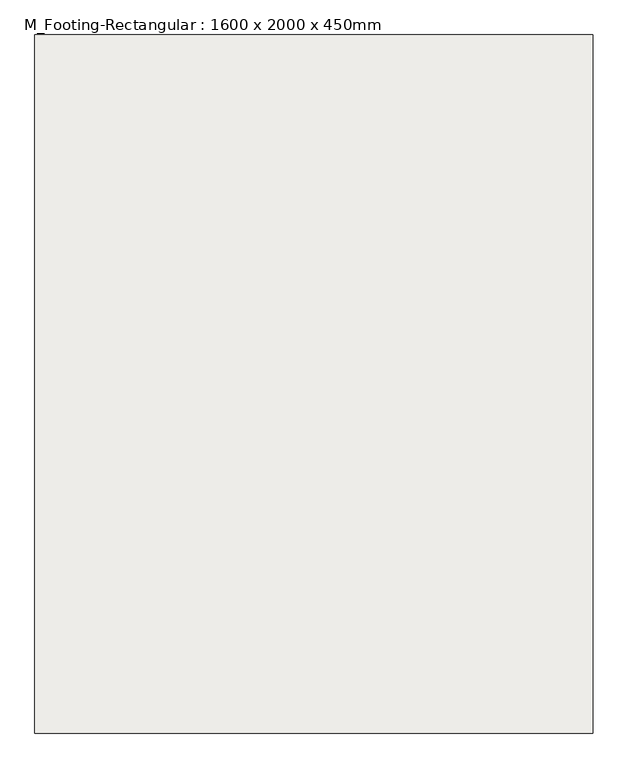
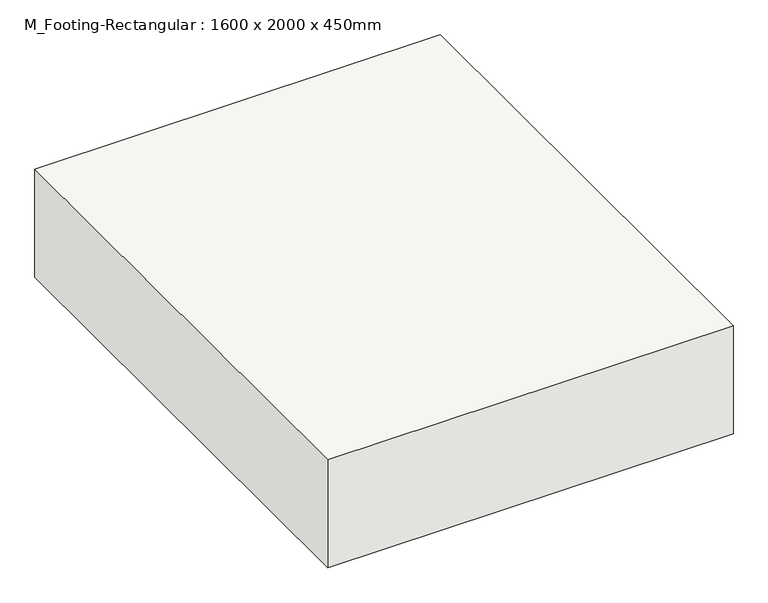
"""IFC4 building model written with IfcOpenShell, lengths in millimetres: slab geometry, M_Footing-Rectangular : 1600 x 2000 x 450mm."""

from ifc_helpers import new_model, si_unit, frame, origin, place, context, project, spatial, polyline, outline, extrude, source, transform, mapped, element, save


def m_footing_rectangular_1600_x_2000_x_450mm_9aacb398(model_context):
    return source(origin(), model_context, "Body", "SweptSolid", [
        extrude(outline(polyline([(800.0, 1000.0), (800.0, -1000.0), (-800.0, -1000.0), (-800.0, 1000.0), (800.0, 1000.0)])), frame((0.0, 0.0, -450.0), z_axis=(0.0, 0.0, 1.0), x_axis=(1.0, 0.0, 0.0)), (0.0, 0.0, 1.0), 450.0),
    ])


if __name__ == "__main__":
    model = new_model("IFC4")
    model_context = context("Model", 3, world=origin())
    ifc_project = project(units=[si_unit("LENGTHUNIT", "METRE", prefix="MILLI")], contexts=[model_context])
    site = spatial("IfcSite", under=ifc_project)
    building = spatial("IfcBuilding", under=site)
    placement = place(None, origin())
    m_footing_rectangular_1600_x_2000_x_450mm_shape = m_footing_rectangular_1600_x_2000_x_450mm_9aacb398(model_context)
    element("IfcSlab", 1, ObjectType="M_Footing-Rectangular : 1600 x 2000 x 450mm", at=placement, inside=building, context=model_context, shape_type="MappedRepresentation", body=[
        mapped(m_footing_rectangular_1600_x_2000_x_450mm_shape, transform((0.0, 0.0, 0.0), x_axis=(1.0, 0.0, 0.0), y_axis=(0.0, 1.0, 0.0), z_axis=(0.0, 0.0, 1.0))),
    ])
    save(model, "model.ifc")

# Revit data of these elements
# Type "M_Footing-Rectangular : 1600 x 2000 x 450mm"
#   Width = 5' - 2.99213"
#   Length = 6' - 6.74016"
#   Foundation Thickness = 1' - 5.71654"
#   Structural Material [instance default] = Concrete, Cast-in-Place gray
#   Assembly Code = ""
# Element 1 (IfcSlab, "M_Footing-Rectangular : 1600 x 2000 x 450mm")
#   Materials on its faces: "Concrete, Cast-in-Place gray"
# Materials
#   "Concrete, Cast-in-Place gray": class "Concrete", colour RGB 192 192 192, transparency 0, Description = "Cast-in-place concrete", Cost = 0
